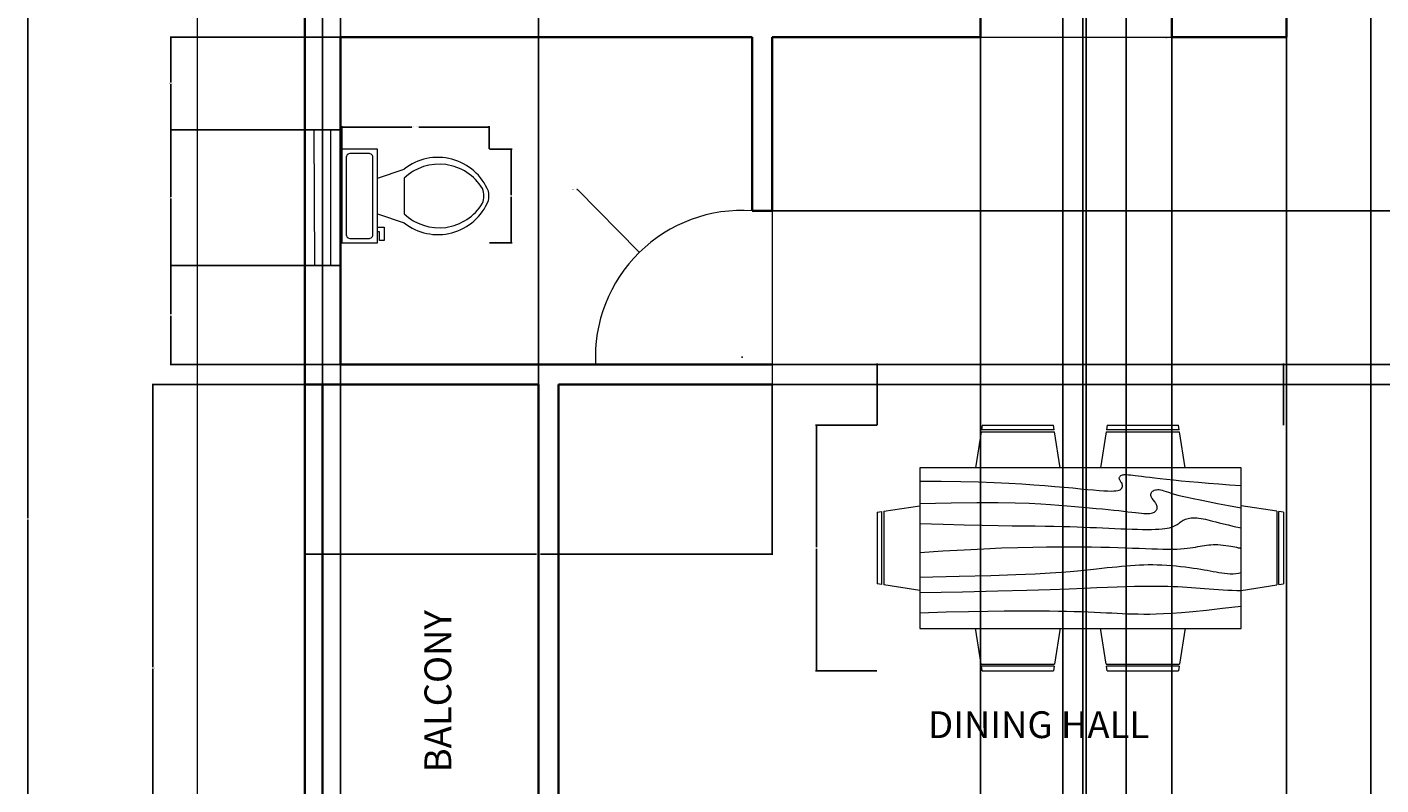
# Model space of a CAD drawing. Units: inches. Extents: x 4700 to 5209, y 8078 to 8754.
# Tile 2 of 5: x 4701 to 5004, y 8356 to 8526. Entities that reach past the tile are written whole.
import ezdxf

# ---------------------------------------------------------------- set-up
doc = ezdxf.new("R2010")
doc.units = ezdxf.units.IN
for name, color, linetype, lineweight in [('A-ANNO-DIMS', 2, 'Continuous', 18), ('A-AREA-IDEN', 7, 'Continuous', 18), ('A-DOOR', 3, 'Continuous', 18), ('A-FLOR-FIXT', 9, 'Continuous', 18), ('A-FURN', 8, 'Continuous', 18), ('A-GLAZ', 4, 'Continuous', 18), ('A-WALL', 7, 'Continuous', 35), ('C-PROP', 8, 'Continuous', 18)]:
    doc.layers.add(name, color=color, linetype=linetype, lineweight=lineweight)
doc.styles.get("Standard").update_dxf_attribs({"font": 'arial.ttf'})
doc.dimstyles.get("Standard").update_dxf_attribs({"dimtxt": 0.18, "dimasz": 0.18, "dimexe": 0.18, "dimexo": 0.0625, "dimgap": 0.09, "dimtad": 0, "dimtih": 1, "dimtoh": 1, "dimdec": 4, "dimzin": 0, "dimdsep": 46, "dimtxsty": 'Standard', "dimcen": 0.09, "dimadec": 0, "dimazin": 0, "dimtfac": 1, "dimtdec": 4, "dimtofl": 0, "dimtmove": 0, "dimatfit": 3, "dimfxl": 1, "dimtolj": 1, "dimtzin": 0, "dimarcsym": 0})

# ---------------------------------------------------------------- blocks, each defined once
blk = doc.blocks.new('Dining Set - 36 x 72 in.')
for p, q in [((-22, 27.5), (-22.1562, 26.50042)), ((-22, 27.5), (-6, 27.5)), ((-5.8437, 26.49966), (-6, 27.5)), ((6, 27.5), (5.8438, 26.50042)), ((6, 27.5), (22, 27.5)), ((22.1563, 26.49966), (22, 27.5)), ((-22.2343, 26.00059), (-23.4847, 17.99762)), ((-22.2304, 26), (-5.7608, 26)), ((-5.8416, 26.5), (-22.1534, 26.5)), ((-4.5152, 17.99762), (-5.7655, 25.99926)), ((5.7657, 26.00059), (4.5153, 17.99762)), ((5.7696, 26), (22.2392, 26)), ((22.1584, 26.5), (5.8466, 26.5)), ((23.4848, 17.99762), (22.2345, 25.99926)), ((36, 18), (-36, 18)), ((-36, 18), (-36, -18)), ((36, -18), (36, 18)), ((-44.0006, 8.23428), (-35.9976, 9.48474)), ((44.0006, 8.23428), (35.9976, 9.48474)), ((-45.5, 8), (-44.5004, 8.15617)), ((-45.5, 8), (-45.5, -8)), ((-44.5, -8.15843), (-44.5, 8.15338)), ((-44, 8.23041), (-44, -8.23915)), ((44, 8.23041), (44, -8.23915)), ((44.5, -8.15843), (44.5, 8.15338)), ((45.5, 8), (44.5005, 8.15617)), ((45.5, 8), (45.5, -8)), ((-44.4997, -8.15631), (-45.5, -8)), ((-35.9976, -9.48476), (-43.9993, -8.2345)), ((35.9976, -9.48476), (43.9993, -8.2345)), ((44.4997, -8.15631), (45.5, -8)), ((-36, -18), (36, -18)), ((-22.2343, -26.0006), (-23.4847, -17.99762)), ((-4.5152, -17.99762), (-5.7655, -25.99928)), ((5.7657, -26.0006), (4.5153, -17.99762)), ((23.4848, -17.99762), (22.2345, -25.99928)), ((-22.2304, -26), (-5.7608, -26)), ((-22, -27.5), (-22.1562, -26.50044)), ((-5.8416, -26.5), (-22.1534, -26.5)), ((-5.8437, -26.49967), (-6, -27.5)), ((5.7696, -26), (22.2392, -26)), ((6, -27.5), (5.8438, -26.50044)), ((22.1584, -26.5), (5.8466, -26.5)), ((22.1563, -26.49967), (22, -27.5)), ((-22, -27.5), (-6, -27.5)), ((6, -27.5), (22, -27.5))]:
    blk.add_line(p, q)
for points in [[(-36, 15), (-31.1772, 14.97754), (-26.8079, 14.91406), (-22.8538, 14.81543), (-19.276, 14.6875), (-16.0362, 14.53613), (-13.0957, 14.36718), (-10.4159, 14.18652), (-7.9583, 14), (-5.6904, 13.81315), (-3.6035, 13.63021), (-1.6954, 13.45508), (0.0365, 13.29166), (1.5945, 13.14388), (2.9811, 13.01562), (4.1988, 12.9108), (5.25, 12.83333), (6.1393, 12.78613), (6.8802, 12.76823), (7.4883, 12.77767), (7.9792, 12.8125), (8.3685, 12.87077), (8.6719, 12.95052), (8.9049, 13.0498), (9.0833, 13.16666), (9.2205, 13.29899), (9.3216, 13.44401), (9.3895, 13.59879), (9.4271, 13.76041), (9.4373, 13.92594), (9.4232, 14.09245), (9.3875, 14.257), (9.3333, 14.41666), (9.2638, 14.56917), (9.1836, 14.71484), (9.0975, 14.85465), (9.0104, 14.98958), (8.9272, 15.1206), (8.8529, 15.2487), (8.7922, 15.37483), (8.75, 15.5), (8.7305, 15.62467), (8.7344, 15.74739), (8.7617, 15.86621), (8.8125, 15.97916), (8.8867, 16.08431), (8.9844, 16.17968), (9.1055, 16.26334), (9.25, 16.33333), (9.4189, 16.38802), (9.6172, 16.42708), (9.8506, 16.45052), (10.125, 16.45833), (10.4463, 16.45052), (10.8203, 16.42708), (11.2529, 16.38802), (11.75, 16.33333), (12.3184, 16.26318), (12.9694, 16.17838), (13.7151, 16.07991), (14.5677, 15.96875), (15.5395, 15.84586), (16.6426, 15.71224), (17.8893, 15.56884), (19.2917, 15.41666), (20.859, 15.25667), (22.5879, 15.08984), (24.4721, 14.91715), (26.5052, 14.73958), (28.6809, 14.5581), (30.9929, 14.3737), (33.4347, 14.18733), (36, 14)], [(-36, 10), (-28.9766, 10.14274), (-23.1725, 10.20442), (-18.4241, 10.19775), (-14.5677, 10.13541), (-11.4399, 10.03011), (-8.877, 9.89453), (-6.7154, 9.74137), (-4.7917, 9.58333), (-2.9698, 9.43082), (-1.2246, 9.28515), (0.4415, 9.14534), (2.026, 9.01041), (3.5266, 8.87939), (4.9408, 8.7513), (6.266, 8.62516), (7.5, 8.5), (8.6411, 8.37549), (9.6914, 8.2539), (10.6538, 8.13818), (11.5312, 8.03125), (12.3267, 7.93603), (13.043, 7.85547), (13.6831, 7.79248), (14.25, 7.75), (14.7471, 7.7303), (15.1797, 7.73307), (15.5537, 7.75732), (15.875, 7.80208), (16.1494, 7.86637), (16.3828, 7.94922), (16.5811, 8.04964), (16.75, 8.16666), (16.8944, 8.29915), (17.0143, 8.44531), (17.1089, 8.60319), (17.1771, 8.77083), (17.218, 8.94629), (17.2305, 9.1276), (17.2137, 9.31282), (17.1667, 9.5), (17.0895, 9.6875), (16.987, 9.875), (16.8649, 10.0625), (16.7292, 10.25), (16.5856, 10.4375), (16.4401, 10.625), (16.2985, 10.8125), (16.1667, 11), (16.05, 11.18733), (15.9518, 11.3737), (15.8752, 11.5581), (15.8229, 11.73958), (15.798, 11.91715), (15.8034, 12.08984), (15.842, 12.25667), (15.9167, 12.41666), (16.0295, 12.56836), (16.1784, 12.70833), (16.3605, 12.83268), (16.5729, 12.9375), (16.8127, 13.01888), (17.0768, 13.07291), (17.3625, 13.0957), (17.6667, 13.08333), (17.9894, 13.03312), (18.3418, 12.94726), (18.7382, 12.82918), (19.1927, 12.68229), (19.7195, 12.51001), (20.3327, 12.31575), (21.0465, 12.10294), (21.875, 11.875), (22.8357, 11.63354), (23.959, 11.37304), (25.2786, 11.08618), (26.8282, 10.76562), (28.6414, 10.40405), (30.752, 9.99414), (33.1936, 9.52856), (36, 9)], [(-36, 5.5), (-30.7157, 5.3348), (-26.069, 5.20963), (-21.9946, 5.11767), (-18.4271, 5.05208), (-15.3009, 5.00602), (-12.5508, 4.97265), (-10.1112, 4.94515), (-7.9167, 4.91666), (-5.909, 4.88167), (-4.0586, 4.83984), (-2.3429, 4.79215), (-0.7396, 4.73958), (0.7739, 4.6831), (2.22, 4.6237), (3.6213, 4.56233), (5, 4.5), (6.373, 4.43782), (7.7344, 4.3776), (9.0723, 4.32129), (10.375, 4.27083), (11.6309, 4.22819), (12.8281, 4.19531), (13.9551, 4.17415), (15, 4.16666), (15.954, 4.17448), (16.819, 4.19791), (17.6001, 4.23698), (18.3021, 4.29166), (18.9299, 4.36198), (19.4883, 4.44791), (19.9823, 4.54948), (20.4167, 4.66666), (20.7969, 4.79899), (21.1302, 4.94401), (21.4245, 5.09879), (21.6875, 5.26041), (21.9271, 5.42594), (22.1511, 5.59245), (22.3672, 5.757), (22.5834, 5.91666), (22.8065, 6.06868), (23.0404, 6.21093), (23.2879, 6.34147), (23.5521, 6.45833), (23.8358, 6.55957), (24.142, 6.64323), (24.4735, 6.70735), (24.8334, 6.75), (25.2235, 6.76969), (25.642, 6.76692), (26.0858, 6.74267), (26.5521, 6.69791), (27.0379, 6.63362), (27.5404, 6.55078), (28.0565, 6.45036), (28.5834, 6.33333), (29.1242, 6.19987), (29.7071, 6.04687), (30.3661, 5.87044), (31.1354, 5.66666), (32.0493, 5.43164), (33.142, 5.16146), (34.4475, 4.85221), (36, 4.5)], [(-36, -1), (-30.7915, -0.6591), (-26.0195, -0.38216), (-21.6519, -0.16284), (-17.6563, 0.00521), (-14.0005, 0.12833), (-10.6523, 0.21289), (-7.5796, 0.26522), (-4.75, 0.29166), (-2.134, 0.29793), (0.2878, 0.28711), (2.5317, 0.26163), (4.6146, 0.22396), (6.5529, 0.17651), (8.3633, 0.12174), (10.0623, 0.06209), (11.6667, 0), (13.1899, -0.06201), (14.6341, -0.1211), (15.9982, -0.17432), (17.2813, -0.21875), (18.4823, -0.25147), (19.6003, -0.26953), (20.6343, -0.27002), (21.5834, -0.25), (22.4481, -0.20768), (23.2357, -0.14584), (23.9549, -0.06836), (24.6146, 0.02083), (25.2235, 0.11784), (25.7904, 0.21875), (26.3241, 0.31966), (26.8334, 0.41666), (27.3265, 0.50618), (27.8099, 0.58593), (28.2894, 0.65397), (28.7709, 0.70833), (29.2601, 0.74707), (29.763, 0.76823), (30.2855, 0.76985), (30.8334, 0.75), (31.4088, 0.70784), (31.9994, 0.64713), (32.589, 0.57275), (33.1615, 0.48958), (33.7008, 0.4025), (34.1908, 0.3164), (34.6153, 0.23616), (34.9584, 0.16666), (35.2099, 0.11165), (35.3848, 0.07031), (35.504, 0.04069), (35.5886, 0.02083), (35.6594, 0.00879), (35.7377, 0.0026), (35.8442, 0.00032), (36, 0)], [(-36, -6.5), (-27.1843, -6.31267), (-20.084, -6.1263), (-14.469, -5.9419), (-10.1094, -5.76042), (-6.7752, -5.58285), (-4.2363, -5.41016), (-2.2629, -5.24333), (-0.625, -5.08334), (0.8708, -4.93099), (2.2715, -4.78646), (3.5872, -4.64974), (4.8281, -4.52084), (6.0046, -4.39974), (7.127, -4.28646), (8.2053, -4.18099), (9.25, -4.08334), (10.2705, -3.99382), (11.2734, -3.91407), (12.2647, -3.84603), (13.25, -3.79167), (14.2354, -3.75293), (15.2266, -3.73177), (16.2295, -3.73015), (17.25, -3.75), (18.2912, -3.79248), (19.3451, -3.85547), (20.4009, -3.93604), (21.4479, -4.03125), (22.4754, -4.13819), (23.4727, -4.25391), (24.4289, -4.37549), (25.3334, -4.5), (26.1785, -4.62492), (26.9694, -4.74935), (27.7145, -4.87281), (28.4219, -4.99479), (29.1, -5.11483), (29.7572, -5.23242), (30.4016, -5.34709), (31.0417, -5.45834), (31.6837, -5.56437), (32.3262, -5.65821), (32.9658, -5.73153), (33.599, -5.77604), (34.2224, -5.78345), (34.8327, -5.74545), (35.4264, -5.65373), (36, -5.5)], [(-36, -10), (-26.4022, -9.81299), (-18.4675, -9.62891), (-11.9839, -9.45069), (-6.7396, -9.28125), (-2.5226, -9.12354), (0.8789, -8.98047), (3.6769, -8.85498), (6.0833, -8.75), (8.2767, -8.66765), (10.3021, -8.60677), (12.1712, -8.56543), (13.8958, -8.54167), (15.4876, -8.53353), (16.9583, -8.53907), (18.3197, -8.55632), (19.5834, -8.58334), (20.7616, -8.61841), (21.8685, -8.66081), (22.9188, -8.71004), (23.9271, -8.76563), (24.9081, -8.82707), (25.8763, -8.89388), (26.8465, -8.96558), (27.8334, -9.04167), (28.8474, -9.12118), (29.8828, -9.20117), (30.93, -9.27824), (31.9792, -9.34896), (33.0205, -9.40991), (34.0443, -9.45768), (35.0407, -9.48885), (36, -9.5)], [(-36, -14.5), (-30.0881, -14.33513), (-25.0332, -14.21224), (-20.7312, -14.12647), (-17.0781, -14.07292), (-13.97, -14.04671), (-11.3027, -14.04297), (-8.9724, -14.05681), (-6.875, -14.08334), (-4.9224, -14.11833), (-3.0905, -14.16016), (-1.3709, -14.20785), (0.2448, -14.26042), (1.7647, -14.3169), (3.1973, -14.3763), (4.5507, -14.43767), (5.8333, -14.5), (7.0554, -14.5621), (8.235, -14.62175), (9.3922, -14.67652), (10.5469, -14.72396), (11.7192, -14.76164), (12.929, -14.78711), (14.1965, -14.79794), (15.5417, -14.79167), (16.9933, -14.76424), (18.6152, -14.70508), (20.4804, -14.60197), (22.6615, -14.44271), (25.2312, -14.21509), (28.2624, -13.9069), (31.8277, -13.50594), (36, -13)]]:
    blk.add_lwpolyline(points)
blk = doc.blocks.new('Toilet - top')
for p, q in [((9.5, -6), (9.5, -2)), ((-10, -8.5), (-8, -8.5)), ((-10, -9.5), (-10, -8.5)), ((-8, -8.5), (-8, -8)), ((-7, -8), (-7, -9.5)), ((-4, -8), (-6, -14)), ((4, -8), (6, -14)), ((-7, -9.5), (-10, -9.5)), ((4, -14), (-4, -14))]:
    blk.add_line(p, q)
blk.add_lwpolyline([(10.5, -8), (10.5, 0), (-10.5, 0), (-10.5, -8)], close=True)
for points in [[(-9.5, -2), (-9.5, -6)], [(8.5, -1), (-8.5, -1)], [(-8.5, -7), (8.5, -7)]]:
    blk.add_lwpolyline(points)
for centre, radius, start, end in [((-8.62, -1.88), 0.884, 81.8699, 188.1301), ((8.62, -1.88), 0.884, 351.8699, 98.1301), ((-8.62, -6.12), 0.884, 171.8699, 278.1301), ((8.62, -6.12), 0.884, 261.8699, 8.1301), ((3.52, -21.58), 12.17, 141.4691, 247.9714), ((4.2, -21.82), 11.33, 136.3677, 238.9468), ((-3.52, -21.58), 12.17, 292.0284, 38.5307), ((-4.2, -21.82), 11.33, 301.053, 43.6321), ((0, -27.88), 4, 245.7318, 294.2682), ((0, -29), 4, 254.8605, 285.1395)]:
    blk.add_arc(centre, radius, start, end)
blk = doc.blocks.new('*D8')
at = {"layer": 'A-ANNO-DIMS', "color": 0, "lineweight": -2, "transparency": 16777216}
for p, q in [((4771.07, 8498.71), (4771.07, 8503.78)), ((4771.25, 8503.6), (4786.82, 8503.6)), ((4803.94, 8503.6), (4788.37, 8503.6)), ((4804.12, 8498.71), (4804.12, 8503.78))]:
    blk.add_line(p, q, dxfattribs=at)
at = {"layer": 'A-ANNO-DIMS', "color": 0, "transparency": 16777216}
for points in [[(4771.25, 8503.63), (4771.25, 8503.57), (4771.07, 8503.6)], [(4803.94, 8503.63), (4803.94, 8503.57), (4804.12, 8503.6)]]:
    blk.add_solid(points, dxfattribs=at)
at = {"layer": 'Defpoints', "color": 0, "transparency": 16777216}
for p in [(4771.07, 8503.6), (4771.07, 8498.65), (4804.12, 8498.65)]:
    blk.add_point(p, dxfattribs=at)
at = {"layer": 'A-ANNO-DIMS', "color": 0, "transparency": 16777216, "insert": (4787.59, 8503.6), "char_height": 0.18, "attachment_point": 5}
blk.add_mtext('\\A1;WC 33 TYP.', dxfattribs=at)
blk = doc.blocks.new('*D9')
at = {"layer": 'A-ANNO-DIMS', "color": 0, "lineweight": -2, "transparency": 16777216}
for p, q in [((4804.18, 8498.65), (4809.25, 8498.65)), ((4809.07, 8498.47), (4809.07, 8488.33)), ((4809.07, 8477.83), (4809.07, 8487.97)), ((4804.18, 8477.65), (4809.25, 8477.65))]:
    blk.add_line(p, q, dxfattribs=at)
at = {"layer": 'A-ANNO-DIMS', "color": 0, "transparency": 16777216}
for points in [[(4809.04, 8498.47), (4809.1, 8498.47), (4809.07, 8498.65)], [(4809.04, 8477.83), (4809.1, 8477.83), (4809.07, 8477.65)]]:
    blk.add_solid(points, dxfattribs=at)
at = {"layer": 'Defpoints', "color": 0, "transparency": 16777216}
for p in [(4804.12, 8498.65), (4809.07, 8498.65), (4804.12, 8477.65)]:
    blk.add_point(p, dxfattribs=at)
at = {"layer": 'A-ANNO-DIMS', "color": 0, "transparency": 16777216, "insert": (4809.07, 8488.15), "char_height": 0.18, "attachment_point": 5}
blk.add_mtext('\\A1;21 TYP.', dxfattribs=at)
blk = doc.blocks.new('*D12')
at = {"layer": 'A-ANNO-DIMS', "color": 0, "lineweight": -2, "transparency": 16777216}
for p, q in [((4891.08, 8436.82), (4891.08, 8450.59)), ((4891.26, 8450.41), (4935.62, 8450.41)), ((4981.9, 8450.41), (4937.53, 8450.41)), ((4982.08, 8436.82), (4982.08, 8450.59))]:
    blk.add_line(p, q, dxfattribs=at)
at = {"layer": 'A-ANNO-DIMS', "color": 0, "transparency": 16777216}
for points in [[(4891.26, 8450.44), (4891.26, 8450.38), (4891.08, 8450.41)], [(4981.9, 8450.44), (4981.9, 8450.38), (4982.08, 8450.41)]]:
    blk.add_solid(points, dxfattribs=at)
at = {"layer": 'Defpoints', "color": 0, "transparency": 16777216}
for p in [(4982.08, 8450.41), (4891.08, 8436.76), (4982.08, 8436.76)]:
    blk.add_point(p, dxfattribs=at)
at = {"layer": 'A-ANNO-DIMS', "color": 0, "transparency": 16777216, "insert": (4936.58, 8450.41), "char_height": 0.18, "attachment_point": 5}
blk.add_mtext('\\A1;DINING SET 91', dxfattribs=at)
blk = doc.blocks.new('*D13')
at = {"layer": 'A-ANNO-DIMS', "color": 0, "lineweight": -2, "transparency": 16777216}
for p, q in [((4891.01, 8436.76), (4877.25, 8436.76)), ((4877.43, 8436.58), (4877.43, 8409.44)), ((4877.43, 8381.94), (4877.43, 8409.08)), ((4891.01, 8381.76), (4877.25, 8381.76))]:
    blk.add_line(p, q, dxfattribs=at)
at = {"layer": 'A-ANNO-DIMS', "color": 0, "transparency": 16777216}
for points in [[(4877.4, 8436.58), (4877.46, 8436.58), (4877.43, 8436.76)], [(4877.4, 8381.94), (4877.46, 8381.94), (4877.43, 8381.76)]]:
    blk.add_solid(points, dxfattribs=at)
at = {"layer": 'Defpoints', "color": 0, "transparency": 16777216}
for p in [(4877.43, 8436.76), (4891.08, 8436.76), (4891.08, 8381.76)]:
    blk.add_point(p, dxfattribs=at)
at = {"layer": 'A-ANNO-DIMS', "color": 0, "transparency": 16777216, "insert": (4877.43, 8409.26), "char_height": 0.18, "attachment_point": 5}
blk.add_mtext('\\A1;55', dxfattribs=at)
blk = doc.blocks.new('*D15')
at = {"layer": 'A-ANNO-DIMS', "color": 0, "lineweight": -2, "transparency": 16777216}
for p, q in [((4738.72, 8715.75), (4700.6, 8715.75)), ((4700.78, 8715.57), (4700.78, 8415.93)), ((4700.78, 8115.93), (4700.78, 8415.57)), ((4738.72, 8115.75), (4700.6, 8115.75))]:
    blk.add_line(p, q, dxfattribs=at)
at = {"layer": 'A-ANNO-DIMS', "color": 0, "transparency": 16777216}
for points in [[(4700.75, 8715.57), (4700.81, 8715.57), (4700.78, 8715.75)], [(4700.75, 8115.93), (4700.81, 8115.93), (4700.78, 8115.75)]]:
    blk.add_solid(points, dxfattribs=at)
at = {"layer": 'Defpoints', "color": 0, "transparency": 16777216}
for p in [(4700.78, 8715.75), (4738.78, 8715.75), (4738.78, 8115.75)]:
    blk.add_point(p, dxfattribs=at)
at = {"layer": 'A-ANNO-DIMS', "color": 0, "transparency": 16777216, "insert": (4700.78, 8415.75), "char_height": 0.18, "attachment_point": 5}
blk.add_mtext('\\A1;600', dxfattribs=at)
blk = doc.blocks.new('*D31')
at = {"layer": 'A-ANNO-DIMS', "color": 0, "lineweight": -2, "transparency": 16777216}
for p, q in [((4766.72, 8445.91), (4728.6, 8445.91)), ((4728.78, 8445.73), (4728.78, 8382.56)), ((4728.78, 8319.03), (4728.78, 8382.19)), ((4766.72, 8318.85), (4728.6, 8318.85))]:
    blk.add_line(p, q, dxfattribs=at)
at = {"layer": 'A-ANNO-DIMS', "color": 0, "transparency": 16777216}
for points in [[(4728.75, 8445.73), (4728.81, 8445.73), (4728.78, 8445.91)], [(4728.75, 8319.03), (4728.81, 8319.03), (4728.78, 8318.85)]]:
    blk.add_solid(points, dxfattribs=at)
at = {"layer": 'Defpoints', "color": 0, "transparency": 16777216}
for p in [(4728.78, 8445.91), (4766.78, 8445.91), (4766.78, 8318.85)]:
    blk.add_point(p, dxfattribs=at)
at = {"layer": 'A-ANNO-DIMS', "color": 0, "transparency": 16777216, "insert": (4728.78, 8382.38), "char_height": 0.18, "attachment_point": 5}
blk.add_mtext('\\A1;127.06', dxfattribs=at)
blk = doc.blocks.new('*D32')
at = {"layer": 'A-ANNO-DIMS', "color": 0, "lineweight": -2, "transparency": 16777216}
for p, q in [((4770.72, 8472.58), (4732.6, 8472.58)), ((4732.78, 8472.4), (4732.78, 8461.67)), ((4732.78, 8450.59), (4732.78, 8461.31)), ((4770.72, 8450.41), (4732.6, 8450.41))]:
    blk.add_line(p, q, dxfattribs=at)
at = {"layer": 'A-ANNO-DIMS', "color": 0, "transparency": 16777216}
for points in [[(4732.75, 8472.4), (4732.81, 8472.4), (4732.78, 8472.58)], [(4732.75, 8450.59), (4732.81, 8450.59), (4732.78, 8450.41)]]:
    blk.add_solid(points, dxfattribs=at)
at = {"layer": 'Defpoints', "color": 0, "transparency": 16777216}
for p in [(4732.78, 8472.58), (4770.78, 8472.58), (4770.78, 8450.41)]:
    blk.add_point(p, dxfattribs=at)
at = {"layer": 'A-ANNO-DIMS', "color": 0, "transparency": 16777216, "insert": (4732.78, 8461.49), "char_height": 0.18, "attachment_point": 5}
blk.add_mtext('\\A1;22.172', dxfattribs=at)
blk = doc.blocks.new('*D33')
at = {"layer": 'A-ANNO-DIMS', "color": 0, "lineweight": -2, "transparency": 16777216}
for p, q in [((4770.72, 8503), (4732.6, 8503)), ((4732.78, 8502.82), (4732.78, 8487.97)), ((4732.78, 8472.76), (4732.78, 8487.61)), ((4770.72, 8472.58), (4732.6, 8472.58))]:
    blk.add_line(p, q, dxfattribs=at)
at = {"layer": 'A-ANNO-DIMS', "color": 0, "transparency": 16777216}
for points in [[(4732.75, 8502.82), (4732.81, 8502.82), (4732.78, 8503)], [(4732.75, 8472.76), (4732.81, 8472.76), (4732.78, 8472.58)]]:
    blk.add_solid(points, dxfattribs=at)
at = {"layer": 'Defpoints', "color": 0, "transparency": 16777216}
for p in [(4732.78, 8503), (4770.78, 8503), (4770.78, 8472.58)]:
    blk.add_point(p, dxfattribs=at)
at = {"layer": 'A-ANNO-DIMS', "color": 0, "transparency": 16777216, "insert": (4732.78, 8487.79), "char_height": 0.18, "attachment_point": 5}
blk.add_mtext('\\A1;30.42', dxfattribs=at)
blk = doc.blocks.new('*D34')
at = {"layer": 'A-ANNO-DIMS', "color": 0, "lineweight": -2, "transparency": 16777216}
for p, q in [((4770.72, 8523.75), (4732.6, 8523.75)), ((4732.78, 8523.57), (4732.78, 8513.56)), ((4732.78, 8503.18), (4732.78, 8513.19)), ((4770.72, 8503), (4732.6, 8503))]:
    blk.add_line(p, q, dxfattribs=at)
at = {"layer": 'A-ANNO-DIMS', "color": 0, "transparency": 16777216}
for points in [[(4732.75, 8523.57), (4732.81, 8523.57), (4732.78, 8523.75)], [(4732.75, 8503.18), (4732.81, 8503.18), (4732.78, 8503)]]:
    blk.add_solid(points, dxfattribs=at)
at = {"layer": 'Defpoints', "color": 0, "transparency": 16777216}
for p in [(4732.78, 8523.75), (4770.78, 8523.75), (4770.78, 8503)]:
    blk.add_point(p, dxfattribs=at)
at = {"layer": 'A-ANNO-DIMS', "color": 0, "transparency": 16777216, "insert": (4732.78, 8513.37), "char_height": 0.18, "attachment_point": 5}
blk.add_mtext('\\A1;20.754', dxfattribs=at)
blk = doc.blocks.new('*D49')
at = {"layer": 'A-ANNO-DIMS', "color": 0, "lineweight": -2, "transparency": 16777216}
for p, q in [((4766.78, 8318.91), (4766.78, 8753.93)), ((4766.96, 8753.75), (4790.57, 8753.75)), ((4814.97, 8753.75), (4791.36, 8753.75)), ((4815.15, 8318.91), (4815.15, 8753.93))]:
    blk.add_line(p, q, dxfattribs=at)
at = {"layer": 'A-ANNO-DIMS', "color": 0, "transparency": 16777216}
for points in [[(4766.96, 8753.78), (4766.96, 8753.72), (4766.78, 8753.75)], [(4814.97, 8753.78), (4814.97, 8753.72), (4815.15, 8753.75)]]:
    blk.add_solid(points, dxfattribs=at)
at = {"layer": 'Defpoints', "color": 0, "transparency": 16777216}
for p in [(4815.15, 8753.75), (4766.78, 8318.85), (4815.15, 8318.85)]:
    blk.add_point(p, dxfattribs=at)
at = {"layer": 'A-ANNO-DIMS', "color": 0, "transparency": 16777216, "insert": (4790.96, 8753.75), "char_height": 0.18, "attachment_point": 5}
blk.add_mtext('\\A1;48.37', dxfattribs=at)
blk = doc.blocks.new('*D50')
at = {"layer": 'A-ANNO-DIMS', "color": 0, "lineweight": -2, "transparency": 16777216}
for p, q in [((4762.78, 8445.84), (4762.78, 8407.73)), ((4867.52, 8445.84), (4867.52, 8407.73)), ((4762.96, 8407.91), (4814.69, 8407.91)), ((4867.34, 8407.91), (4815.6, 8407.91))]:
    blk.add_line(p, q, dxfattribs=at)
at = {"layer": 'A-ANNO-DIMS', "color": 0, "transparency": 16777216}
for points in [[(4762.96, 8407.94), (4762.96, 8407.88), (4762.78, 8407.91)], [(4867.34, 8407.94), (4867.34, 8407.88), (4867.52, 8407.91)]]:
    blk.add_solid(points, dxfattribs=at)
at = {"layer": 'Defpoints', "color": 0, "transparency": 16777216}
for p in [(4762.78, 8445.91), (4867.52, 8445.91), (4762.78, 8407.91)]:
    blk.add_point(p, dxfattribs=at)
at = {"layer": 'A-ANNO-DIMS', "color": 0, "transparency": 16777216, "insert": (4815.15, 8407.91), "char_height": 0.18, "attachment_point": 5}
blk.add_mtext('\\A1;104.74', dxfattribs=at)
blk = doc.blocks.new('*D51')
at = {"layer": 'A-ANNO-DIMS', "color": 0, "lineweight": -2, "transparency": 16777216}
for p, q in [((4770.78, 8207.81), (4770.78, 8753.93)), ((4770.96, 8753.75), (4851.26, 8753.75)), ((4932.47, 8753.75), (4852.17, 8753.75)), ((4932.65, 8207.81), (4932.65, 8753.93))]:
    blk.add_line(p, q, dxfattribs=at)
at = {"layer": 'A-ANNO-DIMS', "color": 0, "transparency": 16777216}
for points in [[(4770.96, 8753.78), (4770.96, 8753.72), (4770.78, 8753.75)], [(4932.47, 8753.78), (4932.47, 8753.72), (4932.65, 8753.75)]]:
    blk.add_solid(points, dxfattribs=at)
at = {"layer": 'Defpoints', "color": 0, "transparency": 16777216}
for p in [(4932.65, 8753.75), (4770.78, 8207.75), (4932.65, 8207.75)]:
    blk.add_point(p, dxfattribs=at)
at = {"layer": 'A-ANNO-DIMS', "color": 0, "transparency": 16777216, "insert": (4851.71, 8753.75), "char_height": 0.18, "attachment_point": 5}
blk.add_mtext('\\A1;161.87', dxfattribs=at)
blk = doc.blocks.new('*D55')
at = {"layer": 'A-ANNO-DIMS', "color": 0, "lineweight": -2, "transparency": 16777216}
for p, q in [((4937.15, 8207.81), (4937.15, 8753.93)), ((4937.33, 8753.75), (4969.02, 8753.75)), ((5001.49, 8753.75), (4969.8, 8753.75)), ((5001.67, 8207.81), (5001.67, 8753.93))]:
    blk.add_line(p, q, dxfattribs=at)
at = {"layer": 'A-ANNO-DIMS', "color": 0, "transparency": 16777216}
for points in [[(4937.33, 8753.78), (4937.33, 8753.72), (4937.15, 8753.75)], [(5001.49, 8753.78), (5001.49, 8753.72), (5001.67, 8753.75)]]:
    blk.add_solid(points, dxfattribs=at)
at = {"layer": 'Defpoints', "color": 0, "transparency": 16777216}
for p in [(5001.67, 8753.75), (4937.15, 8207.75), (5001.67, 8207.75)]:
    blk.add_point(p, dxfattribs=at)
at = {"layer": 'A-ANNO-DIMS', "color": 0, "transparency": 16777216, "insert": (4969.41, 8753.75), "char_height": 0.18, "attachment_point": 5}
blk.add_mtext('\\A1;64.53', dxfattribs=at)
blk = doc.blocks.new('*D62')
at = {"layer": 'A-ANNO-DIMS', "color": 0, "lineweight": -2, "transparency": 16777216}
for p, q in [((4937.87, 8162.31), (4937.87, 8753.93)), ((4938.05, 8753.75), (4942.22, 8753.75)), ((4946.69, 8753.75), (4942.52, 8753.75)), ((4946.87, 8162.31), (4946.87, 8753.93))]:
    blk.add_line(p, q, dxfattribs=at)
at = {"layer": 'A-ANNO-DIMS', "color": 0, "transparency": 16777216}
for points in [[(4938.05, 8753.78), (4938.05, 8753.72), (4937.87, 8753.75)], [(4946.69, 8753.78), (4946.69, 8753.72), (4946.87, 8753.75)]]:
    blk.add_solid(points, dxfattribs=at)
at = {"layer": 'Defpoints', "color": 0, "transparency": 16777216}
for p in [(4946.87, 8753.75), (4937.87, 8162.25), (4946.87, 8162.25)]:
    blk.add_point(p, dxfattribs=at)
at = {"layer": 'A-ANNO-DIMS', "color": 0, "transparency": 16777216, "insert": (4942.37, 8753.75), "char_height": 0.18, "attachment_point": 5}
blk.add_mtext('\\A1;9', dxfattribs=at)
blk = doc.blocks.new('*D63')
at = {"layer": 'A-ANNO-DIMS', "color": 0, "lineweight": -2, "transparency": 16777216}
for p, q in [((4914.2, 8523.69), (4914.2, 8077.57)), ((4957.05, 8523.69), (4957.05, 8077.57)), ((4914.38, 8077.75), (4935.23, 8077.75)), ((4956.87, 8077.75), (4936.02, 8077.75))]:
    blk.add_line(p, q, dxfattribs=at)
at = {"layer": 'A-ANNO-DIMS', "color": 0, "transparency": 16777216}
for points in [[(4914.38, 8077.78), (4914.38, 8077.72), (4914.2, 8077.75)], [(4956.87, 8077.78), (4956.87, 8077.72), (4957.05, 8077.75)]]:
    blk.add_solid(points, dxfattribs=at)
at = {"layer": 'Defpoints', "color": 0, "transparency": 16777216}
for p in [(4914.2, 8523.75), (4957.05, 8523.75), (4957.05, 8077.75)]:
    blk.add_point(p, dxfattribs=at)
at = {"layer": 'A-ANNO-DIMS', "color": 0, "transparency": 16777216, "insert": (4935.63, 8077.75), "char_height": 0.18, "attachment_point": 5}
blk.add_mtext('\\A1;42.85', dxfattribs=at)
blk = doc.blocks.new('*D64')
at = {"layer": 'A-ANNO-DIMS', "color": 0, "lineweight": -2, "transparency": 16777216}
for p, q in [((4982.78, 8523.69), (4982.78, 8077.57)), ((5024.22, 8523.69), (5024.22, 8077.57)), ((4982.96, 8077.75), (5003.1, 8077.75)), ((5024.04, 8077.75), (5003.9, 8077.75))]:
    blk.add_line(p, q, dxfattribs=at)
at = {"layer": 'A-ANNO-DIMS', "color": 0, "transparency": 16777216}
for points in [[(4982.96, 8077.78), (4982.96, 8077.72), (4982.78, 8077.75)], [(5024.04, 8077.78), (5024.04, 8077.72), (5024.22, 8077.75)]]:
    blk.add_solid(points, dxfattribs=at)
at = {"layer": 'Defpoints', "color": 0, "transparency": 16777216}
for p in [(4982.78, 8523.75), (5024.22, 8523.75), (5024.22, 8077.75)]:
    blk.add_point(p, dxfattribs=at)
at = {"layer": 'A-ANNO-DIMS', "color": 0, "transparency": 16777216, "insert": (5003.5, 8077.75), "char_height": 0.18, "attachment_point": 5}
blk.add_mtext('\\A1;41.44', dxfattribs=at)
blk = doc.blocks.new('*D65')
at = {"layer": 'A-ANNO-DIMS', "color": 0, "lineweight": -2, "transparency": 16777216}
for p, q in [((4957.05, 8523.69), (4957.05, 8077.57)), ((4982.78, 8523.69), (4982.78, 8077.57)), ((4957.23, 8077.75), (4969.52, 8077.75)), ((4982.6, 8077.75), (4970.31, 8077.75))]:
    blk.add_line(p, q, dxfattribs=at)
at = {"layer": 'A-ANNO-DIMS', "color": 0, "transparency": 16777216}
for points in [[(4957.23, 8077.78), (4957.23, 8077.72), (4957.05, 8077.75)], [(4982.6, 8077.78), (4982.6, 8077.72), (4982.78, 8077.75)]]:
    blk.add_solid(points, dxfattribs=at)
at = {"layer": 'Defpoints', "color": 0, "transparency": 16777216}
for p in [(4957.05, 8523.75), (4982.78, 8523.75), (4982.78, 8077.75)]:
    blk.add_point(p, dxfattribs=at)
at = {"layer": 'A-ANNO-DIMS', "color": 0, "transparency": 16777216, "insert": (4969.91, 8077.75), "char_height": 0.18, "attachment_point": 5}
blk.add_mtext('\\A1;25.73', dxfattribs=at)
blk = doc.blocks.new('*D70')
at = {"layer": 'A-ANNO-DIMS', "color": 0, "lineweight": -2, "transparency": 16777216}
for p, q in [((4867.58, 8484.83), (5208.96, 8484.83)), ((5208.78, 8484.65), (5208.78, 8467.8)), ((5208.78, 8450.59), (5208.78, 8467.43)), ((4867.58, 8450.41), (5208.96, 8450.41))]:
    blk.add_line(p, q, dxfattribs=at)
at = {"layer": 'A-ANNO-DIMS', "color": 0, "transparency": 16777216}
for points in [[(5208.75, 8484.65), (5208.81, 8484.65), (5208.78, 8484.83)], [(5208.75, 8450.59), (5208.81, 8450.59), (5208.78, 8450.41)]]:
    blk.add_solid(points, dxfattribs=at)
at = {"layer": 'Defpoints', "color": 0, "transparency": 16777216}
for p in [(4867.52, 8484.83), (5208.78, 8484.83), (4867.52, 8450.41)]:
    blk.add_point(p, dxfattribs=at)
at = {"layer": 'A-ANNO-DIMS', "color": 0, "transparency": 16777216, "insert": (5208.78, 8467.62), "char_height": 0.18, "attachment_point": 5}
blk.add_mtext('\\A1;34.42', dxfattribs=at)
blk = doc.blocks.new('*D76')
at = {"layer": 'A-ANNO-DIMS', "color": 0, "lineweight": -2, "transparency": 16777216}
for p, q in [((4867.58, 8450.41), (5208.96, 8450.41)), ((5208.78, 8450.23), (5208.78, 8448.34)), ((4867.58, 8445.91), (5208.96, 8445.91)), ((5208.78, 8446.09), (5208.78, 8447.97))]:
    blk.add_line(p, q, dxfattribs=at)
at = {"layer": 'A-ANNO-DIMS', "color": 0, "transparency": 16777216}
for points in [[(5208.75, 8450.23), (5208.81, 8450.23), (5208.78, 8450.41)], [(5208.75, 8446.09), (5208.81, 8446.09), (5208.78, 8445.91)]]:
    blk.add_solid(points, dxfattribs=at)
at = {"layer": 'Defpoints', "color": 0, "transparency": 16777216}
for p in [(4867.52, 8450.41), (4867.52, 8445.91), (5208.78, 8445.91)]:
    blk.add_point(p, dxfattribs=at)
at = {"layer": 'A-ANNO-DIMS', "color": 0, "transparency": 16777216, "insert": (5208.78, 8448.16), "char_height": 0.18, "attachment_point": 5}
blk.add_mtext('\\A1;4.5', dxfattribs=at)
blk = doc.blocks.new('*D79')
at = {"layer": 'A-ANNO-DIMS', "color": 0, "lineweight": -2, "transparency": 16777216}
for p, q in [((4911.66, 8574.22), (4911.84, 8574.22)), ((4911.84, 8574.22), (4928.21, 8555.41)), ((4955.72, 8523.7), (4955.9, 8523.7)), ((4955.81, 8523.61), (4955.81, 8523.79))]:
    blk.add_line(p, q, dxfattribs=at)
at = {"layer": 'A-ANNO-DIMS', "color": 0, "transparency": 16777216}
blk.add_solid([(4928.24, 8555.43), (4928.19, 8555.39), (4928.33, 8555.28)], dxfattribs=at)
at = {"layer": 'Defpoints', "color": 0, "transparency": 16777216}
for p in [(4928.33, 8555.28), (4955.81, 8523.7)]:
    blk.add_point(p, dxfattribs=at)
at = {"layer": 'A-ANNO-DIMS', "color": 0, "transparency": 16777216, "insert": (4911.18, 8574.22), "char_height": 0.18, "attachment_point": 5}
blk.add_mtext('\\A1;R41.86', dxfattribs=at)
blk = doc.blocks.new('*D82')
at = {"layer": 'A-ANNO-DIMS', "color": 0, "lineweight": -2, "transparency": 16777216}
for p, q in [((4823.75, 8489.57), (4823.93, 8489.57)), ((4823.93, 8489.57), (4837.62, 8475.62)), ((4860.68, 8452.04), (4860.86, 8452.04)), ((4860.77, 8451.95), (4860.77, 8452.13))]:
    blk.add_line(p, q, dxfattribs=at)
at = {"layer": 'A-ANNO-DIMS', "color": 0, "transparency": 16777216}
blk.add_solid([(4837.64, 8475.65), (4837.6, 8475.6), (4837.75, 8475.5)], dxfattribs=at)
at = {"layer": 'Defpoints', "color": 0, "transparency": 16777216}
for p in [(4837.75, 8475.5), (4860.77, 8452.04)]:
    blk.add_point(p, dxfattribs=at)
at = {"layer": 'A-ANNO-DIMS', "color": 0, "transparency": 16777216, "insert": (4823.2, 8489.57), "char_height": 0.18, "attachment_point": 5}
blk.add_mtext('\\A1;R32.867', dxfattribs=at)

msp = doc.modelspace()

# ---------------------------------------------------------------- linework, layer by layer
at = {"layer": 'A-DOOR'}
for p, q in [((4914.2028, 8523.7503), (4957.0498, 8523.7503)), ((4867.5173, 8484.828), (4867.5173, 8445.9056))]:
    msp.add_line(p, q, dxfattribs=at)
msp.add_arc((4860.7683, 8452.0385), 32.8665, 86.076158, 182.84769, dxfattribs=at)
at = {"layer": 'A-GLAZ'}
for p, q in [((4764.8065, 8502.9966), (4764.9898, 8472.5781)), ((4766.7803, 8502.9966), (4766.7803, 8472.5781)), ((4768.5631, 8502.9966), (4768.5631, 8472.5781))]:
    msp.add_line(p, q, dxfattribs=at)
msp.add_lwpolyline([(4762.7803, 8502.9966), (4770.7803, 8502.9966), (4770.7803, 8472.5781), (4762.7803, 8472.5781)], close=True, dxfattribs=at)
at = {"layer": 'A-WALL'}
for p, q in [((4762.7803, 8199.7503), (4762.7803, 8691.7503)), ((4914.2028, 8523.7503), (4914.2028, 8528.2503)), ((4957.0498, 8528.2503), (4957.0498, 8523.7503)), ((4982.778, 8523.7503), (4982.778, 8528.2503)), ((4770.7803, 8523.7503), (4863.0173, 8523.7503)), ((4770.7803, 8450.4056), (4770.7803, 8523.7503)), ((4863.0173, 8484.828), (4863.0173, 8523.7503)), ((4867.5173, 8484.828), (4867.5173, 8523.7503)), ((4867.5173, 8523.7503), (4914.2028, 8523.7503)), ((4957.0498, 8523.7503), (4982.778, 8523.7503)), ((4867.5173, 8484.828), (4863.0173, 8484.828)), ((4863.0173, 8450.4056), (4770.7803, 8450.4056)), ((4863.0173, 8450.4056), (4867.5173, 8450.4056)), ((4770.7803, 8445.9056), (4762.7803, 8445.9056)), ((4766.7803, 8318.8479), (4766.7803, 8445.9056)), ((4815.1488, 8445.9056), (4770.7803, 8445.9056)), ((4815.1488, 8445.9056), (4815.1488, 8318.8479)), ((4867.5173, 8445.9056), (4819.6488, 8445.9056)), ((4819.6488, 8445.9056), (4819.6488, 8318.8479))]:
    msp.add_line(p, q, dxfattribs=at)
at = {"layer": 'C-PROP'}
msp.add_line((4738.7803, 8115.7503), (4738.7803, 8715.7503), dxfattribs=at)

# ---------------------------------------------------------------- block references
at = {"layer": 'A-FLOR-FIXT', "rotation": 90}
msp.add_blockref('Toilet - top', (4771.0713, 8488.1479), dxfattribs=at)
at = {"layer": 'A-FURN'}
msp.add_blockref('Dining Set - 36 x 72 in.', (4936.5759, 8409.2619), dxfattribs=at)

# ---------------------------------------------------------------- texts
at = {"layer": 'A-AREA-IDEN', "insert": (4789.6142, 8358.9868), "char_height": 6, "attachment_point": 1, "rotation": 90}
msp.add_mtext_dynamic_manual_height_columns('BALCONY', width=51.756341, gutter_width=12.5, heights=[0], dxfattribs=at)
at = {"layer": 'A-AREA-IDEN', "insert": (4902.458, 8372.6697), "char_height": 6, "attachment_point": 1}
msp.add_mtext_dynamic_manual_height_columns('DINING HALL', width=69.841054, gutter_width=12.5, heights=[0], dxfattribs=at)

# ---------------------------------------------------------------- dimensions: what is measured, and where the dimension line sits
at = {"layer": 'A-ANNO-DIMS'}
for base, p1, p2, override, picture, middle in [((4815.1488, 8753.7503), (4766.7803, 8318.8479), (4815.1488, 8318.8479), {"dimdec": 2, "dimlfac": 1, "dimrnd": 0, "dimzin": 0, "dimdsep": 46, "dimlunit": 2}, '*D49', (4790.9646, 8753.7503)), ((4932.6464, 8753.7503), (4770.7803, 8207.7503), (4932.6464, 8207.7503), {"dimdec": 2, "dimlfac": 1, "dimrnd": 0, "dimzin": 0, "dimdsep": 46, "dimlunit": 2}, '*D51', (4851.7134, 8753.7503)), ((5001.6744, 8753.7503), (4937.1464, 8207.7503), (5001.6744, 8207.7503), {"dimdec": 2, "dimlfac": 1, "dimrnd": 0, "dimzin": 0, "dimdsep": 46, "dimlunit": 2}, '*D55', (4969.4104, 8753.7503)), ((4946.8701, 8753.7503), (4937.87, 8162.2503), (4946.8701, 8162.2503), {"dimdec": 0, "dimlfac": 1, "dimrnd": 0, "dimzin": 0, "dimdsep": 46, "dimlunit": 2}, '*D62', (4942.3701, 8753.7503)), ((4957.0498, 8077.7503), (4914.2028, 8523.7503), (4957.0498, 8523.7503), {"dimdec": 2, "dimlfac": 1, "dimrnd": 0, "dimzin": 0, "dimdsep": 46, "dimlunit": 2}, '*D63', (4935.6263, 8077.7503)), ((4982.778, 8077.7503), (4957.0498, 8523.7503), (4982.778, 8523.7503), {"dimdec": 2, "dimlfac": 1, "dimrnd": 0, "dimzin": 0, "dimdsep": 46, "dimlunit": 2}, '*D65', (4969.9139, 8077.7503)), ((5024.2192, 8077.7503), (4982.778, 8523.7503), (5024.2192, 8523.7503), {"dimdec": 2, "dimlfac": 1, "dimrnd": 0, "dimzin": 0, "dimdsep": 46, "dimlunit": 2}, '*D64', (5003.4986, 8077.7503))]:
    dim = msp.add_linear_dim(base=base, p1=p1, p2=p2, dimstyle='Standard', override=override, dxfattribs=at)
    dim.commit()
    dim.dimension.update_dxf_attribs({"geometry": picture, "text_midpoint": middle})
for base, p1, p2, angle, override, picture, middle in [((4700.7803, 8715.7503), (4738.7803, 8115.7503), (4738.7803, 8715.7503), 90, {"dimdec": 0, "dimlfac": 1, "dimrnd": 0, "dimzin": 0, "dimdsep": 46, "dimlunit": 2}, '*D15', (4700.7803, 8415.7503)), ((4732.7803, 8523.7503), (4770.7803, 8502.9966), (4770.7803, 8523.7503), 90, {"dimdec": 3, "dimlfac": 1, "dimrnd": 0, "dimzin": 0, "dimdsep": 46, "dimlunit": 2}, '*D34', (4732.7803, 8513.3735)), ((4732.7803, 8502.9966), (4770.7803, 8472.5781), (4770.7803, 8502.9966), 90, {"dimdec": 2, "dimlfac": 1, "dimrnd": 0, "dimzin": 0, "dimdsep": 46, "dimlunit": 2}, '*D33', (4732.7803, 8487.7873)), ((5208.7803, 8484.828), (4867.5173, 8450.4056), (4867.5173, 8484.828), 90, {"dimdec": 2, "dimlfac": 1, "dimrnd": 0, "dimzin": 0, "dimdsep": 46, "dimlunit": 2}, '*D70', (5208.7803, 8467.6168)), ((4732.78033, 8472.57809), (4770.78033, 8450.40565), (4770.78033, 8472.57809), 90, {"dimdec": 3, "dimlfac": 1, "dimrnd": 0, "dimzin": 0, "dimdsep": 46, "dimlunit": 2}, '*D32', (4732.78033, 8461.49187)), ((5208.7803, 8445.9056), (4867.5173, 8450.4056), (4867.5173, 8445.9056), 90, {"dimdec": 1, "dimlfac": 1, "dimrnd": 0, "dimzin": 0, "dimdsep": 46, "dimlunit": 2}, '*D76', (5208.7803, 8448.1556)), ((4728.7803, 8445.9056), (4766.7803, 8318.8479), (4766.7803, 8445.9056), 90, {"dimdec": 2, "dimlfac": 1, "dimrnd": 0, "dimzin": 0, "dimdsep": 46, "dimlunit": 2}, '*D31', (4728.7803, 8382.3768)), ((4762.7803, 8407.9056), (4867.5173, 8445.9056), (4762.7803, 8445.9056), 180, {"dimdec": 2, "dimlfac": 1, "dimrnd": 0, "dimzin": 0, "dimdsep": 46, "dimlunit": 2}, '*D50', (4815.1488, 8407.9056)), ((4877.4259, 8436.7619), (4891.0759, 8381.7619), (4891.0759, 8436.7619), 90, {"dimdec": 0, "dimlfac": 1, "dimrnd": 0, "dimzin": 0, "dimdsep": 46, "dimlunit": 2}, '*D13', (4877.4259, 8409.2619))]:
    dim = msp.add_linear_dim(base=base, p1=p1, p2=p2, angle=angle, dimstyle='Standard', override=override, dxfattribs=at)
    dim.commit()
    dim.dimension.update_dxf_attribs({"geometry": picture, "text_midpoint": middle})
for center, mpoint, override, picture, middle in [((4955.8142, 8523.7042), (4928.332, 8555.278), {"dimdec": 2, "dimlfac": 1, "dimrnd": 0, "dimzin": 0, "dimdsep": 46, "dimlunit": 2}, '*D79', (4911.1829, 8574.2223)), ((4860.76827, 8452.03849), (4837.74726, 8475.49574), {"dimdec": 3, "dimlfac": 1, "dimrnd": 0, "dimzin": 0, "dimdsep": 46, "dimlunit": 2}, '*D82', (4823.20489, 8489.57009))]:
    dim = msp.add_radius_dim(center=center, mpoint=mpoint, dimstyle='Standard', override=override, dxfattribs=at)
    dim.commit()
    dim.dimension.update_dxf_attribs({"geometry": picture, "text_midpoint": middle, "dimtype": 164})
for base, p1, p2, angle, text, picture, middle in [((4771.0713, 8503.6048), (4804.1175, 8498.6479), (4771.0713, 8498.6479), 180, 'WC <> TYP.', '*D8', (4787.5944, 8503.6048)), ((4809.0745, 8498.6479), (4804.1175, 8477.6479), (4804.1175, 8498.6479), 90, '<> TYP.', '*D9', (4809.0745, 8488.1479))]:
    dim = msp.add_linear_dim(base=base, p1=p1, p2=p2, angle=angle, text=text, dimstyle='Standard', override={"dimdec": 0, "dimlfac": 1, "dimrnd": 0, "dimzin": 0, "dimdsep": 46, "dimlunit": 2}, dxfattribs=at)
    dim.commit()
    dim.dimension.update_dxf_attribs({"geometry": picture, "text_midpoint": middle})
dim = msp.add_linear_dim(base=(4982.0759, 8450.4119), p1=(4891.0759, 8436.7619), p2=(4982.0759, 8436.7619), text='DINING SET <>', dimstyle='Standard', override={"dimdec": 0, "dimlfac": 1, "dimrnd": 0, "dimzin": 0, "dimdsep": 46, "dimlunit": 2}, dxfattribs=at)
dim.commit()
dim.dimension.update_dxf_attribs({"geometry": '*D12', "text_midpoint": (4936.5759, 8450.4119)})

doc.saveas('drawing.dxf')
